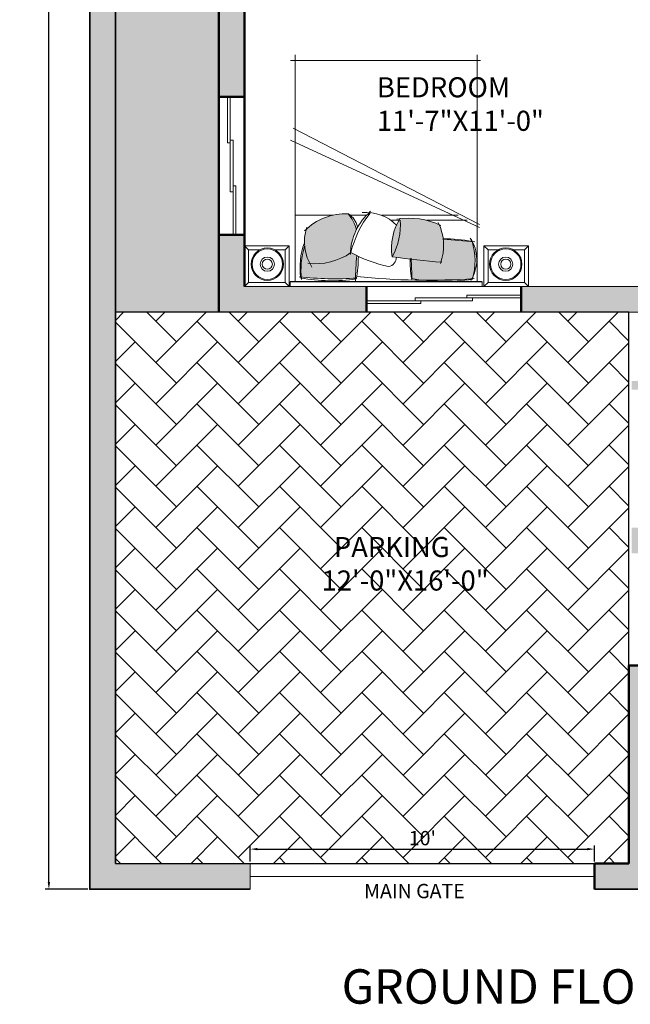
# Model space of a CAD drawing. Units: inches. Extents: x 1734 to 4011, y 1071 to 1891.
# Tile 14 of 27: x 3092 to 3304, y 1072 to 1415. Entities that reach past the tile are written whole.
import ezdxf

# ---------------------------------------------------------------- set-up
doc = ezdxf.new("R2010")
doc.units = ezdxf.units.IN
for name, color, linetype, lineweight in [('0.10', 252, 'Continuous', 9), ('0.15', 34, 'Continuous', 15), ('A-ANNO-DIMS', 2, 'Continuous', 18), ('A-ANNO-TEXT', 7, 'Continuous', 25), ('A-AREA-IDEN', 3, 'Continuous', 18), ('A-FLOR-OTLN', 7, 'Continuous', 25), ('A-FLOR-PATT', 252, 'Continuous', 13), ('A-FURN', 8, 'Continuous', 18), ('A-FURN-PATT', 252, 'Continuous', 13), ('A-GLAZ', 4, 'Continuous', 18), ('A-WALL', 7, 'Continuous', 50), ('A-WALL-PATT', 8, 'Continuous', 13), ('C-PROP', 1, 'Continuous', 35)]:
    doc.layers.add(name, color=color, linetype=linetype, lineweight=lineweight)
doc.styles.get("Standard").update_dxf_attribs({"font": 'arial.ttf'})
doc.dimstyles.new('ISO-25', dxfattribs={"dimtxt": 5, "dimasz": 2.5, "dimexe": 1.25, "dimexo": 0.625, "dimtad": 1, "dimdec": 1, "dimlunit": 3, "dimtxsty": 'Standard', "dimcen": 2.5, "dimclrt": 1, "dimadec": 0, "dimazin": 0, "dimtfac": 1, "dimtdec": 1, "dimtmove": 0, "dimatfit": 3, "dimfxl": 1, "dimarcsym": 0})

# ---------------------------------------------------------------- blocks, each defined once
blk = doc.blocks.new('*D65')
at = {"layer": 'A-ANNO-DIMS', "color": 0, "lineweight": -2, "transparency": 16777216}
for p, q in [((3171.99, 1121.44), (3171.99, 1127.05)), ((3174.49, 1125.8), (3289.49, 1125.8)), ((3291.99, 1121.44), (3291.99, 1127.05))]:
    blk.add_line(p, q, dxfattribs=at)
at = {"layer": 'A-ANNO-DIMS', "color": 0, "transparency": 16777216}
for points in [[(3174.49, 1126.22), (3174.49, 1125.39), (3171.99, 1125.8)], [(3289.49, 1126.22), (3289.49, 1125.39), (3291.99, 1125.8)]]:
    blk.add_solid(points, dxfattribs=at)
at = {"layer": 'Defpoints', "color": 0, "transparency": 16777216}
for p in [(3291.99, 1125.8), (3171.99, 1120.82), (3291.99, 1120.82)]:
    blk.add_point(p, dxfattribs=at)
at = {"layer": 'A-ANNO-DIMS', "color": 0, "transparency": 16777216, "insert": (3231.99, 1128.98), "char_height": 5, "attachment_point": 5}
blk.add_mtext("10'", dxfattribs=at)
blk = doc.blocks.new('*D66')
at = {"layer": 'A-ANNO-DIMS', "color": 0, "lineweight": -2, "transparency": 16777216}
for p, q in [((3115.37, 1831.82), (3100.52, 1831.82)), ((3101.77, 1114.32), (3101.77, 1829.32)), ((3115.37, 1111.82), (3100.52, 1111.82))]:
    blk.add_line(p, q, dxfattribs=at)
at = {"layer": 'A-ANNO-DIMS', "color": 0, "transparency": 16777216}
for points in [[(3101.36, 1829.32), (3102.19, 1829.32), (3101.77, 1831.82)], [(3101.36, 1114.32), (3102.19, 1114.32), (3101.77, 1111.82)]]:
    blk.add_solid(points, dxfattribs=at)
at = {"layer": 'Defpoints', "color": 0, "transparency": 16777216}
for p in [(3101.77, 1831.82), (3115.99, 1831.82), (3115.99, 1111.82)]:
    blk.add_point(p, dxfattribs=at)
at = {"layer": 'A-ANNO-DIMS', "color": 0, "transparency": 16777216, "insert": (3096.55, 1471.82), "char_height": 5, "attachment_point": 5, "rotation": 90}
blk.add_mtext("{\\H1.8x;60'}", dxfattribs=at)
blk = doc.blocks.new('camita')
at = {"layer": '0.10'}
for p, q in [((-0.85, -0.045), (0.85, -0.045)), ((-0.805, -0.045), (-0.805, -2.0485)), ((0.805, -0.045), (0.805, -2.0485)), ((-0.8271, -0.521), (0.8464, -1.2932)), ((-0.8271, -0.5476), (0.8236, -1.3992)), ((-0.7161, -0.585), (-0.3554, -0.585)), ((-0.1136, -0.585), (-0.0485, -0.585)), ((-0.638, -0.63), (0.0434, -0.63)), ((0.1749, -0.63), (0.3179, -0.63)), ((0.4739, -0.63), (0.805, -0.63)), ((-0.8354, -2), (0.8464, -2))]:
    blk.add_line(p, q, dxfattribs=at)
blk.add_lwpolyline([(-0.85, -0.0405), (0.85, -0.0405), (0.85, 0), (-0.85, 0)], close=True, dxfattribs=at)
for centre, radius, start, end in [((-0.4574, -0.2364), 0.3443, 147.50996, 213.83359), ((-0.1997, -0.2266), 0.5864, 163.92635, 197.14087), ((-0.3639, -5.8457), 5.7909, 83.80731, 94.12107), ((-0.5104, -1.7232), 1.6781, 80.12554, 98.66187), ((2.3534, -0.0532), 2.5803, 180.10628, 184.38541), ((-1.5443, -0.2452), 1.3333, 359.93941, 7.55329), ((1.5815, -0.2893), 1.3353, 170.38021, 178.99138), ((-1.4396, -0.0609), 1.7117, 352.92911, 0.39592), ((0.4524, -3.0675), 2.9996, 83.90257, 93.67595), ((0.4863, -1.6286), 1.5781, 80.16015, 98.05996), ((0.0294, -0.1377), 0.7262, 342.58415, 6.00484), ((0.1326, -0.1696), 0.6307, 339.92303, 8.74334), ((0.3203, -0.3944), 0.4043, 341.45245, 33.45121), ((-0.0543, -0.3633), 0.4542, 159.30257, 206.50263), ((-1.3301, -9.6748), 9.4985, 82.27078, 84.93989), ((-0.007, -0.258), 0.0828, 100.01798, 179.73597), ((-0.2931, -1.4378), 1.2903, 61.97485, 77.84351), ((0.6265, -0.7518), 0.5508, 82.96906, 124.67388), ((0.4585, -0.5454), 0.5842, 151.04555, 184.14969), ((-0.5341, -0.3393), 0.4875, 327.26442, 9.0473), ((-0.1986, -0.2742), 0.5159, 310.73945, 359.05759), ((-0.5673, -0.0868), 0.9057, 321.69527, 346.46261), ((-1.8672, -14.986), 14.6323, 84.65974, 85.75157), ((-0.4598, 1.4861), 1.9092, 260.95299, 268.65169), ((0.5707, -0.4317), 0.3145, 192.93877, 221.96363), ((0.3612, -0.133), 0.5096, 267.25889, 315.29965), ((-0.2002, 0.064), 0.6673, 244.78094, 279.06058), ((0.179, -0.272), 0.3828, 224.52836, 275.22287), ((0.4384, -0.4834), 0.1898, 193.68485, 236.70352)]:
    blk.add_arc(centre, radius, start, end, dxfattribs=at)
blk = doc.blocks.new('VELADOR')
at = {"layer": '0.15'}
for p, q in [((-0.248, 0), (-0.203, -0.045)), ((0.248, 0), (0.202, -0.045)), ((-0.203, -0.405), (-0.248, -0.45)), ((0.248, -0.45), (0.202, -0.405))]:
    blk.add_line(p, q, dxfattribs=at)
blk.add_lwpolyline([(-0.248, 0), (-0.248, -0.45), (0.248, -0.45), (0.248, 0)], close=True, dxfattribs=at)
blk.add_lwpolyline([(0.092, -0.405), (0.202, -0.405), (0.202, -0.045), (-0.203, -0.045), (-0.203, -0.405), (-0.082, -0.405)], dxfattribs=at)
for radius in [0.18, 0.169, 0.0788, 0.0563]:
    blk.add_circle((0.005, -0.247), radius, dxfattribs=at)

msp = doc.modelspace()

# ---------------------------------------------------------------- hatches: boundary and pattern name
at = {"layer": 'A-FLOR-PATT'}
h = msp.add_hatch(color=256, dxfattribs=at)
h.dxf.hatch_style = 1
h.paths.add_polyline_path([(3124.99, 1745.82), (3115.99, 1745.82), (3115.99, 1111.82), (3171.99, 1111.82), (3171.99, 1120.82), (3124.99, 1120.82)])
h = msp.add_hatch(color=256, dxfattribs=at)
h.dxf.hatch_style = 1
h.paths.add_polyline_path([(3160.99, 1745.82), (3124.99, 1745.82), (3124.99, 1312.82), (3160.99, 1312.82), (3160.99, 1529.82)])
h = msp.add_hatch(dxfattribs=at)
h.set_pattern_fill('AR-HBONE', color=256, scale=0.1)
h.set_pattern_definition([(45, (1357.344, -12.241), (0, 14.36841), [30.48, -10.16]), (135, (1364.528, -5.057), (1e-15, 14.36841), [30.48, -10.16])])
h.paths.add_polyline_path([(3303.99, 1312.82), (3124.99, 1312.82), (3124.99, 1120.82), (3303.99, 1120.82)])
h.paths.add_polyline_path([(3225.98, 1123.78), (3237.58, 1123.78), (3237.58, 1134.09), (3225.98, 1134.09)], flags=24)
h.paths.add_polyline_path([(3194.05, 1211.9), (3253.89, 1211.9), (3253.89, 1238.02), (3194.05, 1238.02)], flags=24)
at = {"layer": 'A-FURN-PATT'}
h = msp.add_hatch(color=256, dxfattribs=at)
h.dxf.hatch_style = 1
h.paths.add_polyline_path([(3208.99, 1341.59, 0.127326), (3206.13, 1347.1, 0.202559), (3191.46, 1341.72, 0.194952), (3192.74, 1329.82, 0.173835), (3206.91, 1333.49, -0.104045)])
h.paths.add_polyline_path([(3209.19, 1332.51, -0.011742), (3207.06, 1333.59, -0.175864), (3192.74, 1329.82, -0.098488), (3190.93, 1335.77, 0.094792), (3189.71, 1325.09, 0.040212), (3208.68, 1324.71, -0.029051)])
h.paths.add_polyline_path([(3237.9, 1343.33, 0.134508), (3224.16, 1345.39, 0.181694), (3221.46, 1332.16, 0.011408), (3238.42, 1330.25, 0.189536)])
h.paths.add_polyline_path([(3249.36, 1337.39, -0.004387), (3239.28, 1338.25, -0.113891), (3238.42, 1330.25, -0.006967), (3228.05, 1331.32, -0.016701), (3228.32, 1324.54, 0.015442), (3232.36, 1323.98, 0.01851), (3249.23, 1324.5, 0.020657), (3249.74, 1325.5, 0.131047)])
at = {"layer": 'A-WALL-PATT'}
h = msp.add_hatch(color=256, dxfattribs=at)
h.dxf.hatch_style = 1
h.paths.add_polyline_path([(3475.99, 1831.82), (3115.99, 1831.82), (3115.99, 1745.82), (3130.99, 1745.82), (3130.99, 1750.82), (3124.99, 1750.82), (3124.99, 1822.82), (3214.99, 1822.82), (3214.99, 1780.82), (3219.99, 1780.82), (3219.99, 1822.82), (3308.99, 1822.82), (3308.99, 1750.82), (3254.99, 1750.82), (3254.99, 1745.82), (3308.99, 1745.82), (3308.99, 1604.82), (3313.99, 1604.82), (3313.99, 1745.82), (3366.99, 1745.82), (3366.99, 1750.82), (3313.99, 1750.82), (3313.99, 1822.82), (3401.99, 1822.82), (3401.99, 1750.82), (3396.99, 1750.82), (3396.99, 1745.82), (3411.99, 1745.82), (3411.99, 1750.82), (3406.99, 1750.82), (3406.99, 1822.82), (3466.99, 1822.82), (3466.99, 1750.82), (3441.99, 1750.82), (3441.99, 1745.82), (3466.99, 1745.82), (3466.99, 1517.82), (3452.49, 1517.82), (3452.49, 1512.82), (3466.99, 1512.82), (3466.99, 1458.82), (3446.49, 1458.82), (3446.49, 1453.82), (3466.99, 1453.82), (3466.99, 1237.82), (3372.99, 1237.82), (3372.99, 1228.82), (3466.99, 1228.82), (3466.99, 1120.82), (3309.99, 1120.82), (3309.99, 1184.82), (3310.99, 1184.82), (3310.99, 1189.82), (3303.99, 1189.82), (3303.99, 1120.82), (3291.99, 1120.82), (3291.99, 1111.82), (3475.99, 1111.82)])
h.paths.add_polyline_path([(3169.99, 1745.82), (3224.99, 1745.82), (3224.99, 1750.82), (3154.99, 1750.82), (3154.99, 1745.82), (3160.99, 1745.82), (3160.99, 1636.82), (3169.99, 1636.82)], flags=17)
h.paths.add_polyline_path([(3169.99, 1588.82), (3160.99, 1588.82), (3160.99, 1559.82), (3313.99, 1559.82), (3313.99, 1568.82), (3308.99, 1568.82), (3308.99, 1564.82), (3169.99, 1564.82)], flags=17)
h.paths.add_polyline_path([(3416.49, 1517.82), (3401.99, 1517.82), (3401.99, 1512.82), (3416.49, 1512.82)], flags=17)
h.paths.add_polyline_path([(3371.99, 1517.82), (3366.99, 1517.82), (3366.99, 1453.82), (3392.49, 1453.82), (3392.49, 1458.82), (3371.99, 1458.82)], flags=17)
h.paths.add_polyline_path([(3258.99, 1529.82), (3160.99, 1529.82), (3160.99, 1494.82), (3169.99, 1494.82), (3169.99, 1524.82), (3253.99, 1524.82), (3253.99, 1520.82), (3258.99, 1520.82)], flags=17)
h.paths.add_polyline_path([(3263.99, 1458.82), (3258.99, 1458.82), (3258.99, 1490.82), (3253.99, 1490.82), (3253.99, 1458.82), (3169.99, 1458.82), (3169.99, 1470.82), (3160.99, 1470.82), (3160.99, 1387.82), (3169.99, 1387.82), (3169.99, 1453.82), (3263.99, 1453.82)], flags=17)
h.paths.add_polyline_path([(3313.99, 1453.82), (3318.99, 1453.82), (3318.99, 1458.82), (3299.99, 1458.82), (3299.99, 1453.82), (3308.99, 1453.82), (3308.99, 1321.82), (3266.49, 1321.82), (3266.49, 1312.82), (3313.99, 1312.82)], flags=17)
h.paths.add_polyline_path([(3212.49, 1321.82), (3169.99, 1321.82), (3169.99, 1339.82), (3160.99, 1339.82), (3160.99, 1312.82), (3212.49, 1312.82)], flags=17)
h.paths.add_polyline_path([(3313.99, 1288.82), (3304.99, 1288.82), (3304.99, 1285.82), (3313.99, 1285.82)], flags=17)
h.paths.add_polyline_path([(3324.99, 1237.82), (3304.99, 1237.82), (3304.99, 1228.82), (3324.99, 1228.82)], flags=17)

# ---------------------------------------------------------------- linework, layer by layer
at = {"layer": 'A-FLOR-OTLN'}
msp.add_lwpolyline([(3303.99, 1312.82), (3124.99, 1312.82), (3124.99, 1120.82), (3303.99, 1120.82)], close=True, dxfattribs=at)
at = {"layer": 'A-FURN'}
for p, q in [((3169.99, 1321.82), (3308.99, 1321.82)), ((3124.99, 1312.82), (3313.99, 1312.82)), ((3171.99, 1120.82), (3124.99, 1120.82)), ((3171.99, 1120.82), (3171.99, 1111.82)), ((3171.99, 1116.32), (3291.99, 1116.32))]:
    msp.add_line(p, q, dxfattribs=at)
at = {"layer": 'A-GLAZ'}
for p, q in [((3163.99, 1387.82), (3163.99, 1371.82)), ((3164.99, 1387.82), (3164.99, 1354.82)), ((3164.99, 1372.82), (3165.99, 1372.82)), ((3165.99, 1372.82), (3165.99, 1339.82)), ((3163.99, 1371.82), (3164.99, 1371.82)), ((3165.99, 1356.82), (3166.99, 1356.82)), ((3166.99, 1356.82), (3166.99, 1339.82)), ((3164.99, 1354.82), (3165.99, 1354.82)), ((3229.49, 1317.82), (3229.49, 1316.82)), ((3229.49, 1317.82), (3266.49, 1317.82)), ((3247.49, 1318.82), (3247.49, 1317.82)), ((3247.49, 1318.82), (3266.49, 1318.82)), ((3249.49, 1317.82), (3249.49, 1316.82)), ((3212.49, 1316.82), (3249.49, 1316.82)), ((3212.49, 1315.82), (3231.49, 1315.82)), ((3231.49, 1316.82), (3231.49, 1315.82))]:
    msp.add_line(p, q, dxfattribs=at)
at = {"layer": 'A-WALL'}
for p, q in [((3160.99, 1312.82), (3160.99, 1529.82)), ((3169.99, 1321.82), (3169.99, 1453.82)), ((3160.99, 1387.82), (3169.99, 1387.82)), ((3160.99, 1339.82), (3169.99, 1339.82)), ((3212.49, 1321.82), (3212.49, 1312.82)), ((3266.49, 1321.82), (3266.49, 1312.82)), ((3303.99, 1189.82), (3303.99, 1120.82)), ((3310.99, 1189.82), (3303.99, 1189.82)), ((3291.99, 1120.82), (3291.99, 1111.82)), ((3303.99, 1120.82), (3291.99, 1120.82))]:
    msp.add_line(p, q, dxfattribs=at)
at = {"layer": 'C-PROP'}
msp.add_line((3124.99, 1120.82), (3124.99, 1745.82), dxfattribs=at)
msp.add_lwpolyline([(3171.99, 1111.82), (3115.99, 1111.82), (3115.99, 1831.82), (3475.99, 1831.82), (3475.99, 1111.82), (3291.99, 1111.82)], dxfattribs=at)

# ---------------------------------------------------------------- block references
at = {"layer": 'A-FURN', "rotation": 180}
for name, p, xscale, yscale, zscale in [('camita', (3219.39, 1321.82), 39.375, 39.375, 39.375), ('VELADOR', (3177.77, 1321.82), -31.41542173157097, 31.41542173157097, 31.41542173157097), ('VELADOR', (3261.22, 1321.82), 31.41542173157097, 31.41542173157097, 31.41542173157097)]:
    msp.add_blockref(name, p, dxfattribs=dict(at, xscale=xscale, yscale=yscale, zscale=zscale))

# ---------------------------------------------------------------- texts
at = {"layer": 'A-ANNO-TEXT', "attachment_point": 1}
for s, width, insert, char_height in [('MAIN GATE', 86.9528, (3211.68, 1113.69), 5), ('GROUND FLOOR PLAN', 228.5661, (3203.84, 1083.95), 12)]:
    msp.add_mtext_dynamic_manual_height_columns(s, width=width, gutter_width=12.5, heights=[0], dxfattribs=dict(at, insert=insert, char_height=char_height))
at = {"layer": 'A-AREA-IDEN', "char_height": 7, "attachment_point": 1}
for s, insert in [('BEDROOM\\P11\'-7"X11\'-0"', (3216.12, 1394.69)), ('  PARKING\\P12\'-0"X16\'-0"', (3196.86, 1234.54))]:
    msp.add_mtext_dynamic_manual_height_columns(s, width=86.9528, gutter_width=12.5, heights=[0], dxfattribs=dict(at, insert=insert))

# ---------------------------------------------------------------- dimensions: what is measured, and where the dimension line sits
at = {"layer": 'A-ANNO-DIMS'}
dim = msp.add_linear_dim(base=(3101.77, 1831.82), p1=(3115.99, 1111.82), p2=(3115.99, 1831.82), angle=90, text='{\\H1.8x;<>}', dimstyle='ISO-25', override={"dimclrd": 0, "dimclre": 0, "dimclrt": 0}, dxfattribs=at)
dim.commit()
dim.dimension.update_dxf_attribs({"geometry": '*D66', "text_midpoint": (3096.55, 1471.82)})
dim = msp.add_linear_dim(base=(3291.99, 1125.8), p1=(3171.99, 1120.82), p2=(3291.99, 1120.82), dimstyle='ISO-25', override={"dimclrd": 0, "dimclre": 0, "dimclrt": 0}, dxfattribs=at)
dim.commit()
dim.dimension.update_dxf_attribs({"geometry": '*D65', "text_midpoint": (3231.99, 1128.98)})

doc.saveas('drawing.dxf')
